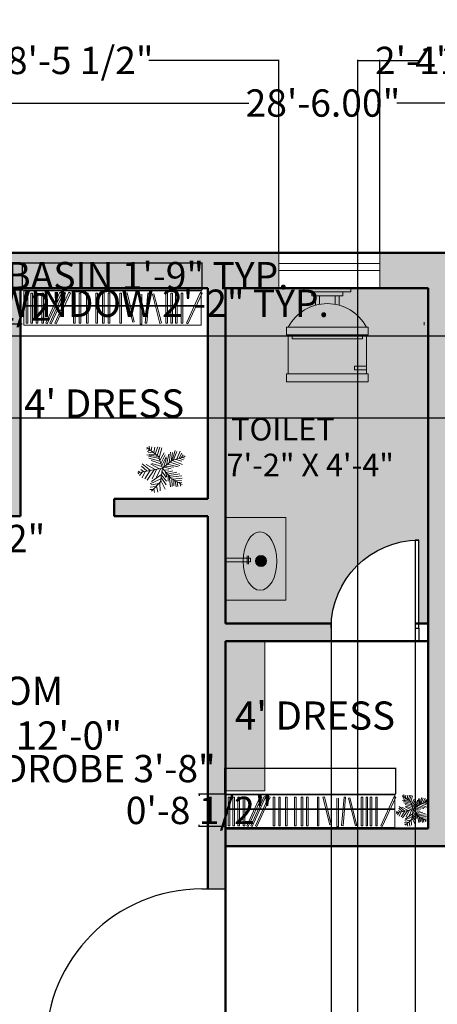
# Model space of a CAD drawing. Units: inches. Extents: x 2974 to 3443, y 2405 to 2963.
# Tile 12 of 13: x 3136 to 3243, y 2711 to 2963. Entities that reach past the tile are written whole.
import ezdxf

# ---------------------------------------------------------------- set-up
doc = ezdxf.new("R2010")
doc.units = ezdxf.units.IN
doc.header["$MEASUREMENT"] = 0
doc.layers.get('0').update_dxf_attribs({"color": 251})
for name, color, linetype, lineweight in [('A-ANNO-DIMS', 2, 'Continuous', 18), ('A-AREA-IDEN', 250, 'Continuous', 25), ('A-DOOR', 32, 'Continuous', 25), ('A-FLOR-CASE-PATT', 9, 'Continuous', 13), ('A-FLOR-FIXT', 8, 'Continuous', 20), ('A-FLOR-FIXT-PATT', 254, 'Continuous', 13), ('A-FLOR-PATT', 9, 'Continuous', 13), ('A-WALL-PATT', 252, 'Continuous', 13), ('closet', 32, 'Continuous', 20), ('greenary', 106, 'Continuous', 13), ('walls', 250, 'Continuous', 50), ('windows', 159, 'Continuous', 20)]:
    doc.layers.add(name, color=color, linetype=linetype, lineweight=lineweight)
doc.styles.get("Standard").update_dxf_attribs({"font": 'arial.ttf'})
doc.dimstyles.get("Standard").update_dxf_attribs({"dimtxt": 7, "dimasz": 0.18, "dimexe": 0.18, "dimexo": 0.0625, "dimgap": 0.09, "dimtad": 0, "dimtih": 1, "dimtoh": 1, "dimzin": 0, "dimdsep": 46, "dimlunit": 3, "dimtxsty": 'Standard', "dimcen": 0.09, "dimadec": 0, "dimazin": 0, "dimtfac": 1, "dimtofl": 0, "dimtmove": 0, "dimatfit": 3, "dimfxl": 1, "dimtolj": 1, "dimtzin": 0, "dimarcsym": 0})

# ---------------------------------------------------------------- blocks, each defined once
blk = doc.blocks.new('*U2')
for p, q in [((0, 0), (0, -6)), ((40, 0), (40, -6))]:
    blk.add_line(p, q)
blk.add_lwpolyline([(0, 0), (0, 40), (1.75, 40), (1.75, 0)], close=True)
blk.add_arc((0, 0), 40, 0, 90)
blk = doc.blocks.new('closet')
at = {"layer": 'closet'}
for p, q in [((-0.71, -5.58), (5.59, 8.19)), ((-0.23, 7.39), (-0.23, -6.57)), ((6.27, 7.88), (-0.04, -5.89)), ((5.59, 8.19), (6.27, 7.88)), ((7.92, 7.84), (8.68, 7.84)), ((7.92, 7.84), (7.92, -5.51)), ((8.68, 7.84), (8.68, -5.51)), ((10.44, 7.84), (11.2, 7.84)), ((10.44, 7.84), (10.44, -5.51)), ((11.2, 7.84), (11.2, -5.51)), ((12.45, 7.84), (13.21, 7.84)), ((12.45, 7.84), (12.45, -5.51)), ((13.21, 7.84), (13.21, -5.51)), ((14.71, 7.84), (15.47, 7.84)), ((14.71, 7.84), (14.71, -5.51)), ((15.47, 7.84), (15.47, -5.51)), ((17.44, 7.75), (18.17, 7.93)), ((17.44, 7.75), (20.73, -5.2)), ((18.17, 7.93), (21.46, -5.01)), ((23.92, 7.84), (22.75, -5.46)), ((24.67, 7.78), (23.51, -5.53)), ((23.92, 7.84), (24.67, 7.78)), ((26.09, 8.25), (26.09, -5.1)), ((26.84, 8.25), (26.84, -5.1)), ((29.49, 7.29), (32.64, -5.69)), ((30.22, 7.46), (33.37, -5.51)), ((35.23, 7.84), (35.23, -5.51)), ((35.99, 7.84), (35.99, -5.51)), ((40.33, 7.84), (40.33, -5.51)), ((41.08, 7.84), (41.08, -5.51)), ((42.85, 7.84), (42.85, -5.51)), ((43.61, 7.84), (43.61, -5.51)), ((45.9, 7.84), (45.9, -5.51)), ((46.65, 7.84), (46.65, -5.51)), ((50.07, 7.84), (50.07, -5.51)), ((50.82, 7.84), (50.82, -5.51)), ((53.32, 7.84), (53.32, -5.51)), ((54.08, 7.84), (54.08, -5.51)), ((55.9, 7.84), (55.9, -5.51)), ((56.65, 7.84), (56.65, -5.51)), ((57.99, -5.58), (64.3, 8.19)), ((64.97, 7.88), (58.67, -5.89)), ((60.19, -5.58), (66.49, 8.19)), ((67.17, 7.88), (60.87, -5.89)), ((62, -5.58), (68.3, 8.19)), ((68.98, 7.88), (62.67, -5.89)), ((69.96, 7.84), (69.96, -5.51)), ((70.72, 7.84), (70.72, -5.51)), ((72.43, 7.84), (72.43, -5.51)), ((73.19, 7.84), (73.19, -5.51)), ((74.82, 7.84), (74.82, -5.51)), ((75.57, 7.84), (75.57, -5.51)), ((76.94, 7.84), (76.94, -5.51)), ((77.69, 7.84), (77.69, -5.51)), ((56.23, 0.33), (0, 0.33)), ((56.2, 0), (0, 0)), ((56.2, 0), (78.76, 0)), ((56.23, 0.33), (78.76, 0.33)), ((-0.04, -5.89), (-0.71, -5.58)), ((21.46, -5.01), (20.73, -5.2)), ((23.51, -5.53), (22.75, -5.46)), ((33.37, -5.51), (32.64, -5.69)), ((35.99, -5.51), (35.23, -5.51)), ((41.08, -5.51), (40.33, -5.51)), ((43.61, -5.51), (42.85, -5.51)), ((46.65, -5.51), (45.9, -5.51)), ((50.82, -5.51), (50.07, -5.51)), ((54.08, -5.51), (53.32, -5.51)), ((56.65, -5.51), (55.9, -5.51)), ((58.67, -5.89), (57.99, -5.58)), ((60.87, -5.89), (60.19, -5.58)), ((62.67, -5.89), (62, -5.58)), ((70.72, -5.51), (69.96, -5.51)), ((73.19, -5.51), (72.43, -5.51)), ((75.57, -5.51), (74.82, -5.51)), ((77.69, -5.51), (76.94, -5.51))]:
    blk.add_line(p, q, dxfattribs=at)
blk = doc.blocks.new('rotated closet')
at = {"layer": 'closet'}
for p, q in [((26.32, 0.86), (27.07, 0.86)), ((29.72, -0.11), (30.45, 0.07)), ((35.46, 0.45), (36.22, 0.45)), ((40.56, 0.45), (41.31, 0.45)), ((43.08, 0.45), (43.84, 0.45)), ((46.13, 0.45), (46.88, 0.45)), ((50.3, 0.45), (51.05, 0.45)), ((53.56, 0.45), (54.31, 0.45)), ((56.13, 0.45), (56.88, 0.45)), ((64.53, 0.8), (65.2, 0.49)), ((66.72, 0.8), (67.4, 0.49)), ((68.53, 0.8), (69.21, 0.49)), ((70.19, 0.45), (70.95, 0.45)), ((72.66, 0.45), (73.42, 0.45)), ((75.05, 0.45), (75.81, 0.45)), ((77.17, 0.45), (77.92, 0.45)), ((78.99, 0), (78.99, -13.96)), ((8.91, -12.91), (8.15, -12.91)), ((11.43, -12.91), (10.67, -12.91)), ((13.44, -12.91), (12.68, -12.91)), ((15.7, -12.91), (14.94, -12.91)), ((-0.46, -14.27), (79.54, -14.27)), ((0, -13.96), (78.99, -13.96))]:
    blk.add_line(p, q, dxfattribs=at)
blk.add_blockref('closet', (0.23, -7.39), dxfattribs=at)
blk = doc.blocks.new('*U18')
for p, q in [((-10, 22), (-10, 12)), ((-10, 21), (-7, 21)), ((-7, 21), (-7, 20)), ((10, 12), (10, 22)), ((-7, 20), (-10, 20)), ((9, 13), (-9, 13)), ((-9, 13), (-9, 12)), ((9, 12), (9, 13)), ((10.5, 12), (-10.5, 12)), ((-10.5, 10), (-10.5, 12)), ((10.5, 12), (10.5, 10)), ((10.5, 10), (-10.5, 10)), ((-3, 4.4065), (-3, 2)), ((-2, 2), (-2, 4.1658)), ((2, 4.1658), (2, 2)), ((3, 2), (3, 4.4065)), ((4, 2), (-4, 2)), ((-4, 2), (-4, 1)), ((4, 1), (4, 2))]:
    blk.add_line(p, q)
for points in [[(10.5, 22), (10.5, 24), (-10.5, 24), (-10.5, 22)], [(6, 0), (6, 1), (-6, 1), (-6, 0)]]:
    blk.add_lwpolyline(points, close=True)
blk.add_arc((0, 15.3333), 11.3333, 208.0725, 331.9275)
blk = doc.blocks.new('*U13')
for p, q in [((-7.288, 39.707), (-21.778, 46.673)), ((-8.737, 47.138), (-17.069, 52.711)), ((-10.186, 53.64), (-13.084, 55.962)), ((0, 0), (-10.5, 57)), ((-9.099, 51.782), (-6.563, 55.962)), ((-7.65, 43.423), (-2.578, 49.46)), ((-5.839, 35.992), (4.667, 48.067)), ((-5.114, 27.632), (10.463, 46.673)), ((-31.5, 4.5), (-52.5, 25.5)), ((-48.585, 21.131), (-49.309, 29.026)), ((-43.513, 28.561), (-42.427, 15.558)), ((-38.442, 26.239), (-34.819, 7.663)), ((-35.544, 28.097), (-24.314, 3.947)), ((-14.533, 2.09), (-30.834, 25.31)), ((-3.665, 19.273), (-27.574, 35.527)), ((-5.114, 28.097), (-24.676, 40.636)), ((-24.314, 23.917), (-2.941, 13.7)), ((-2.941, 16.486), (8.652, 37.85)), ((-1.129, 6.734), (9.014, 26.704)), ((3.942, 1.625), (11.187, 24.381)), ((10.101, 3.483), (17.708, 26.239)), ((16.259, 5.805), (23.142, 31.348)), ((22.055, 7.198), (27.489, 32.277)), ((27, 9), (48, 36)), ((27.127, 9.056), (31.112, 35.992)), ((31.836, 30.883), (32.561, 16.486)), ((35.096, 32.741), (37.27, 22.524)), ((38.719, 34.134), (41.979, 28.561)), ((40.53, 25.775), (48.862, 24.846)), ((43.791, 29.954), (51.036, 30.883)), ((44.153, 36.456), (45.239, 32.741)), ((-47.498, 19.737), (-55.83, 18.344)), ((-40.615, 13.7), (-55.105, 10.913)), ((-33.37, 6.269), (-52.207, 5.34)), ((-28.299, 3.483), (-47.86, -5.805)), ((-21.416, 3.018), (-38.079, -8.128)), ((0, 0), (-31.5, 4.5)), ((-15.982, 2.09), (-30.11, -9.521)), ((0, 0), (-22.5, -19.5)), ((-6.563, 1.161), (-21.416, -8.128)), ((-20.691, 13.7), (-1.129, 4.876)), ((0, 0), (27, 9)), ((0, 0), (18, -22.5)), ((6.478, 1.625), (26.04, -8.592)), ((11.187, 3.483), (30.749, -5.805)), ((18.07, 5.805), (35.096, -3.483)), ((24.229, 7.663), (46.688, 1.625)), ((29.662, 12.307), (48.137, 6.269)), ((33.285, 16.486), (48.862, 10.913)), ((36.183, 19.737), (48.137, 17.88)), ((-17.431, -15.094), (-42.789, -18.809)), ((-24.314, -21.596), (-42.427, -22.06)), ((-22.5, -19.5), (-37.5, -45)), ((-15.257, -12.772), (-30.11, -12.772)), ((-20.691, -18.345), (-17.793, -44.352)), ((-6.563, -5.805), (-19.967, -9.985)), ((-17.069, -15.094), (-12.721, -40.172)), ((-13.446, -11.378), (-8.737, -32.741)), ((-9.461, -8.592), (-6.201, -23.453)), ((-4.752, -3.483), (-3.665, -14.629)), ((2.493, -3.019), (-1.491, -20.202)), ((1.769, -2.555), (24.229, -9.521)), ((5.029, -6.27), (2.131, -25.775)), ((9.014, -11.378), (3.58, -35.992)), ((14.085, -16.951), (6.478, -40.172)), ((7.565, -9.056), (32.198, -14.629)), ((18.07, -22.524), (8.289, -45.745)), ((12.274, -15.094), (36.907, -18.809)), ((16.259, -19.738), (36.183, -22.989)), ((18, -22.5), (27, -52.5)), ((18.433, -22.524), (40.53, -29.026)), ((-28.299, -29.026), (-42.789, -31.348)), ((-30.834, -34.135), (-42.427, -35.528)), ((-34.457, -39.708), (-40.978, -42.494)), ((-26.849, -26.24), (-40.253, -25.775)), ((-32.646, -36.921), (-31.921, -44.352)), ((-29.023, -30.884), (-27.936, -43.887)), ((-25.038, -23.918), (-22.865, -45.281)), ((20.244, -30.419), (15.897, -44.816)), ((19.157, -25.311), (38.719, -33.206)), ((22.78, -37.85), (19.519, -48.532)), ((21.331, -32.741), (39.081, -40.636)), ((22.78, -38.314), (34.372, -44.816)), ((24.591, -43.423), (30.749, -47.603)), ((24.591, -45.745), (23.142, -50.854)), ((26.764, -49.925), (28.213, -50.854))]:
    blk.add_line(p, q)
blk = doc.blocks.new('*D19')
at = {"layer": 'A-ANNO-DIMS', "color": 0, "lineweight": -2, "transparency": 16777216}
for p, q in [((3042.33, 2937.52), (3042.33, 2941.76)), ((3384.33, 2937.52), (3384.33, 2941.76)), ((3042.51, 2941.58), (3194.36, 2941.58)), ((3384.15, 2941.58), (3232.3, 2941.58))]:
    blk.add_line(p, q, dxfattribs=at)
at = {"layer": 'A-ANNO-DIMS', "color": 0, "transparency": 16777216}
for points in [[(3042.51, 2941.61), (3042.51, 2941.55), (3042.33, 2941.58)], [(3384.15, 2941.61), (3384.15, 2941.55), (3384.33, 2941.58)]]:
    blk.add_solid(points, dxfattribs=at)
at = {"layer": 'Defpoints', "color": 0, "transparency": 16777216}
for p in [(3384.33, 2941.58), (3042.33, 2937.45), (3384.33, 2937.45)]:
    blk.add_point(p, dxfattribs=at)
at = {"layer": 'A-ANNO-DIMS', "color": 0, "transparency": 16777216, "insert": (3213.33, 2941.58), "char_height": 7, "attachment_point": 5}
blk.add_mtext('\\A1;28\'-6.00"', dxfattribs=at)
blk = doc.blocks.new('WIN-BATH-26IN')
for p, q in [((0, 0), (0, -9)), ((25.96, 0), (0, 0)), ((0, 0), (0, -2.72)), ((25.96, -9), (25.96, 0)), ((0, -2.72), (25.96, -2.72)), ((25.96, -4.5), (0, -4.5)), ((25.96, -2.72), (25.96, -4.5)), ((0, -9), (25.96, -9))]:
    blk.add_line(p, q)
blk = doc.blocks.new('LAVATORY-WITH-TAP')
h = blk.add_hatch(color=256)
h.dxf.hatch_style = 1
edge = h.paths.add_edge_path()
edge.add_line((0.14, 0.2), (21.04, 0.2))
edge.add_line((21.04, 0.2), (21.04, 15.46))
edge.add_line((21.04, 15.46), (10.75, 15.46))
edge.add_line((10.75, 15.46), (10.75, 10.85))
edge.add_ellipse((10.01, 6.56), major_axis=(-7.48, -0.02), ratio=0.576535, start_angle=272.6137, end_angle=620.1108, ccw=False)
edge.add_line((9.8, 10.87), (9.8, 15.46))
edge.add_line((9.8, 15.46), (0.14, 15.46))
edge.add_line((0.14, 15.46), (0.14, 0.2))
h = blk.add_hatch(color=256)
h.dxf.hatch_style = 1
edge = h.paths.add_edge_path()
edge.add_ellipse((10.01, 6.56), major_axis=(-7.48, -0.02), ratio=0.576535, start_angle=272.6137, end_angle=260.1108)
edge.add_line((10.75, 10.85), (10.75, 9.83))
edge.add_line((10.75, 9.83), (11.35, 9.83))
edge.add_line((11.35, 9.83), (11.35, 9.53))
edge.add_line((11.35, 9.53), (10.75, 9.53))
edge.add_line((10.75, 9.53), (10.75, 9.04))
edge.add_line((10.75, 9.04), (9.8, 9.04))
edge.add_line((9.8, 9.04), (9.8, 10.87))
h.paths.add_polyline_path([(8.24, 6.32, -1), (11.81, 6.32, -1)], flags=16)
h.paths.add_polyline_path([(11.45, 6.32, -1), (8.6, 6.32, -1)], flags=0)
h.paths.add_polyline_path([(8.6, 6.32, 1), (11.45, 6.32, 1)], flags=0)
edge = h.paths.add_edge_path()
edge.add_line((9.8, 9.83), (10.75, 9.83))
edge.add_line((10.75, 9.83), (10.75, 10.85))
edge.add_ellipse((10.01, 6.56), major_axis=(-7.48, -0.02), ratio=0.576535, start_angle=260.1108, end_angle=272.6137)
edge.add_line((9.8, 10.87), (9.8, 9.83))
h.paths.add_polyline_path([(9.8, 9.04), (10.75, 9.04), (10.75, 9.53), (9.8, 9.53)], flags=17)
h.paths.add_polyline_path([(9.8, 9.53), (10.75, 9.53), (10.75, 9.83), (9.8, 9.83)], flags=17)
h.paths.add_polyline_path([(10.75, 9.53), (11.35, 9.53), (11.35, 9.83), (10.75, 9.83)], flags=17)
edge = h.paths.add_edge_path()
edge.add_ellipse((10.01, 6.56), major_axis=(-7.48, -0.02), ratio=0.576535, start_angle=260.1108, end_angle=272.6137, ccw=False)
edge.add_line((10.75, 10.85), (10.75, 15.46))
edge.add_line((10.75, 15.46), (9.8, 15.46))
edge.add_line((9.8, 15.46), (9.8, 10.87))
h = blk.add_hatch(color=256)
h.dxf.hatch_style = 1
h.paths.add_polyline_path([(11.45, 6.32, 1), (8.6, 6.32, 1)], flags=0)
h.paths.add_polyline_path([(11.81, 6.32, 1), (8.24, 6.32, 1)])
h.paths.add_polyline_path([(11.45, 6.32, -1), (8.6, 6.32, -1)], flags=16)
h = blk.add_hatch(color=256)
h.dxf.hatch_style = 1
h.paths.add_polyline_path([(11.45, 6.32, 1), (8.6, 6.32, 1)])
for p, q in [((0, 15.44), (0, 0)), ((9.8, 9.04), (9.8, 15.46)), ((10.75, 9.04), (10.75, 15.46)), ((21.16, 0), (21.16, 15.46)), ((9.22, 9.83), (11.35, 9.83)), ((11.35, 9.53), (9.22, 9.53)), ((9.8, 9.04), (10.75, 9.04)), ((0, 0), (21.16, 0))]:
    blk.add_line(p, q)
blk.add_circle((10.02, 6.32), 1.43)
blk.add_ellipse((10.01, 6.56), major_axis=(-7.48, -0.02), ratio=0.576535)
blk = doc.blocks.new('*D25')
at = {"layer": 'A-ANNO-DIMS', "color": 0, "lineweight": -2, "transparency": 16777216}
for p, q in [((3136.34, 2900.56), (3136.16, 2900.56)), ((3136.34, 2893.72), (3136.34, 2900.74)), ((3182.19, 2900.56), (3136.52, 2900.56)), ((3182.37, 2893.72), (3182.37, 2900.74))]:
    blk.add_line(p, q, dxfattribs=at)
at = {"layer": 'A-ANNO-DIMS', "color": 0, "transparency": 16777216}
for points in [[(3136.52, 2900.59), (3136.52, 2900.53), (3136.34, 2900.56)], [(3182.19, 2900.59), (3182.19, 2900.53), (3182.37, 2900.56)]]:
    blk.add_solid(points, dxfattribs=at)
at = {"layer": 'Defpoints', "color": 0, "transparency": 16777216}
for p in [(3136.34, 2900.56), (3136.34, 2893.66), (3182.37, 2893.66)]:
    blk.add_point(p, dxfattribs=at)
at = {"layer": 'A-ANNO-DIMS', "color": 0, "transparency": 16777216, "insert": (3093.75, 2900.56), "char_height": 7, "attachment_point": 5}
blk.add_mtext('\\A1;WARDROBE 3\'-10"', dxfattribs=at)
blk = doc.blocks.new('*D26')
at = {"layer": 'A-ANNO-DIMS', "color": 0, "lineweight": -2, "transparency": 16777216}
for p, q in [((3136.28, 2893.66), (3129.26, 2893.66)), ((3129.44, 2893.48), (3129.44, 2893.01)), ((3136.28, 2884.95), (3129.26, 2884.95)), ((3129.44, 2885.13), (3129.44, 2885.59))]:
    blk.add_line(p, q, dxfattribs=at)
at = {"layer": 'A-ANNO-DIMS', "color": 0, "transparency": 16777216}
for points in [[(3129.41, 2893.48), (3129.47, 2893.48), (3129.44, 2893.66)], [(3129.41, 2885.13), (3129.47, 2885.13), (3129.44, 2884.95)]]:
    blk.add_solid(points, dxfattribs=at)
at = {"layer": 'Defpoints', "color": 0, "transparency": 16777216}
for p in [(3136.34, 2893.66), (3129.44, 2884.95), (3136.34, 2884.95)]:
    blk.add_point(p, dxfattribs=at)
at = {"layer": 'A-ANNO-DIMS', "color": 0, "transparency": 16777216, "insert": (3129.44, 2889.3), "char_height": 7, "attachment_point": 5}
blk.add_mtext('\\A1;0\'-8 1/2"', dxfattribs=at)
blk = doc.blocks.new('*D28')
at = {"layer": 'A-ANNO-DIMS', "color": 0, "lineweight": -2, "transparency": 16777216}
for p, q in [((3111.77, 2835.69), (3120.92, 2835.69)), ((3120.74, 2835.51), (3120.74, 2833.71)), ((3120.74, 2824.49), (3120.74, 2826.29)), ((3111.77, 2824.31), (3120.92, 2824.31))]:
    blk.add_line(p, q, dxfattribs=at)
at = {"layer": 'A-ANNO-DIMS', "color": 0, "transparency": 16777216}
for points in [[(3120.71, 2835.51), (3120.77, 2835.51), (3120.74, 2835.69)], [(3120.71, 2824.49), (3120.77, 2824.49), (3120.74, 2824.31)]]:
    blk.add_solid(points, dxfattribs=at)
at = {"layer": 'Defpoints', "color": 0, "transparency": 16777216}
for p in [(3111.71, 2835.69), (3111.71, 2824.31), (3120.74, 2824.31)]:
    blk.add_point(p, dxfattribs=at)
at = {"layer": 'A-ANNO-DIMS', "color": 0, "transparency": 16777216, "insert": (3120.74, 2830), "char_height": 7, "attachment_point": 5}
blk.add_mtext('\\A1;0\'-11 1/2"', dxfattribs=at)
blk = doc.blocks.new('*D29')
at = {"layer": 'A-ANNO-DIMS', "color": 0, "lineweight": -2, "transparency": 16777216}
for p, q in [((3188.17, 2771.05), (3187.99, 2771.05)), ((3188.17, 2764.54), (3188.17, 2771.23)), ((3231.81, 2771.05), (3188.35, 2771.05)), ((3231.99, 2764.54), (3231.99, 2771.23))]:
    blk.add_line(p, q, dxfattribs=at)
at = {"layer": 'A-ANNO-DIMS', "color": 0, "transparency": 16777216}
for points in [[(3188.35, 2771.08), (3188.35, 2771.02), (3188.17, 2771.05)], [(3231.81, 2771.08), (3231.81, 2771.02), (3231.99, 2771.05)]]:
    blk.add_solid(points, dxfattribs=at)
at = {"layer": 'Defpoints', "color": 0, "transparency": 16777216}
for p in [(3188.17, 2771.05), (3188.17, 2764.48), (3231.99, 2764.48)]:
    blk.add_point(p, dxfattribs=at)
at = {"layer": 'A-ANNO-DIMS', "color": 0, "transparency": 16777216, "insert": (3148.3, 2771.05), "char_height": 7, "attachment_point": 5}
blk.add_mtext('\\A1;WARDROBE 3\'-8"', dxfattribs=at)
blk = doc.blocks.new('*D30')
at = {"layer": 'A-ANNO-DIMS', "color": 0, "lineweight": -2, "transparency": 16777216}
for p, q in [((3188.11, 2764.48), (3181.42, 2764.48)), ((3181.6, 2764.3), (3181.6, 2764.04)), ((3188.11, 2756.19), (3181.42, 2756.19)), ((3181.6, 2756.37), (3181.6, 2756.62))]:
    blk.add_line(p, q, dxfattribs=at)
at = {"layer": 'A-ANNO-DIMS', "color": 0, "transparency": 16777216}
for points in [[(3181.57, 2764.3), (3181.63, 2764.3), (3181.6, 2764.48)], [(3181.57, 2756.37), (3181.63, 2756.37), (3181.6, 2756.19)]]:
    blk.add_solid(points, dxfattribs=at)
at = {"layer": 'Defpoints', "color": 0, "transparency": 16777216}
for p in [(3188.17, 2764.48), (3181.6, 2756.19), (3188.17, 2756.19)]:
    blk.add_point(p, dxfattribs=at)
at = {"layer": 'A-ANNO-DIMS', "color": 0, "transparency": 16777216, "insert": (3181.6, 2760.33), "char_height": 7, "attachment_point": 5}
blk.add_mtext('\\A1;0\'-8 1/2"', dxfattribs=at)
blk = doc.blocks.new('*D37')
at = {"layer": 'A-ANNO-DIMS', "color": 0, "lineweight": -2, "transparency": 16777216}
for p, q in [((3074.3, 2894.13), (3074.3, 2890.11)), ((3100.26, 2894.13), (3100.26, 2890.11)), ((3074.48, 2890.29), (3100.08, 2890.29)), ((3100.26, 2890.29), (3100.44, 2890.29))]:
    blk.add_line(p, q, dxfattribs=at)
at = {"layer": 'A-ANNO-DIMS', "color": 0, "transparency": 16777216}
for points in [[(3074.48, 2890.32), (3074.48, 2890.26), (3074.3, 2890.29)], [(3100.08, 2890.32), (3100.08, 2890.26), (3100.26, 2890.29)]]:
    blk.add_solid(points, dxfattribs=at)
at = {"layer": 'Defpoints', "color": 0, "transparency": 16777216}
for p in [(3074.3, 2894.19), (3100.26, 2894.19), (3100.26, 2890.29)]:
    blk.add_point(p, dxfattribs=at)
at = {"layer": 'A-ANNO-DIMS', "color": 0, "transparency": 16777216, "insert": (3158.92, 2890.29), "char_height": 7, "attachment_point": 5}
blk.add_mtext('\\A1;BATH WINDOW 2\'-2" TYP.', dxfattribs=at)
blk = doc.blocks.new('*D41')
at = {"layer": 'A-ANNO-DIMS', "color": 0, "lineweight": -2, "transparency": 16777216}
for p, q in [((3109.7, 2894.25), (3109.7, 2897.54)), ((3109.88, 2897.36), (3130.68, 2897.36)), ((3130.86, 2894.25), (3130.86, 2897.54)), ((3130.86, 2897.36), (3131.04, 2897.36))]:
    blk.add_line(p, q, dxfattribs=at)
at = {"layer": 'A-ANNO-DIMS', "color": 0, "transparency": 16777216}
for points in [[(3109.88, 2897.39), (3109.88, 2897.33), (3109.7, 2897.36)], [(3130.68, 2897.39), (3130.68, 2897.33), (3130.86, 2897.36)]]:
    blk.add_solid(points, dxfattribs=at)
at = {"layer": 'Defpoints', "color": 0, "transparency": 16777216}
for p in [(3130.86, 2897.36), (3109.7, 2894.19), (3130.86, 2894.19)]:
    blk.add_point(p, dxfattribs=at)
at = {"layer": 'A-ANNO-DIMS', "color": 0, "transparency": 16777216, "insert": (3168.34, 2897.36), "char_height": 7, "attachment_point": 5}
blk.add_mtext('\\A1;BASIN 1\'-9" TYP.', dxfattribs=at)
blk = doc.blocks.new('*D52')
at = {"layer": 'A-ANNO-DIMS', "color": 0, "lineweight": -2, "transparency": 16777216}
for p, q in [((3100.26, 2903.25), (3100.26, 2952.68)), ((3100.44, 2952.5), (3133.57, 2952.5)), ((3201.81, 2952.5), (3168.68, 2952.5)), ((3201.99, 2903.25), (3201.99, 2952.68))]:
    blk.add_line(p, q, dxfattribs=at)
at = {"layer": 'A-ANNO-DIMS', "color": 0, "transparency": 16777216}
for points in [[(3100.44, 2952.53), (3100.44, 2952.47), (3100.26, 2952.5)], [(3201.81, 2952.53), (3201.81, 2952.47), (3201.99, 2952.5)]]:
    blk.add_solid(points, dxfattribs=at)
at = {"layer": 'Defpoints', "color": 0, "transparency": 16777216}
for p in [(3201.99, 2952.5), (3100.26, 2903.19), (3201.99, 2903.19)]:
    blk.add_point(p, dxfattribs=at)
at = {"layer": 'A-ANNO-DIMS', "color": 0, "transparency": 16777216, "insert": (3151.13, 2952.5), "char_height": 7, "attachment_point": 5}
blk.add_mtext('\\A1;8\'-5 1/2"', dxfattribs=at)
blk = doc.blocks.new('*D53')
at = {"layer": 'A-ANNO-DIMS', "color": 0, "lineweight": -2, "transparency": 16777216}
for p, q in [((3227.95, 2903.25), (3227.95, 2952.68)), ((3228.13, 2952.5), (3238.07, 2952.5)), ((3283.38, 2952.5), (3273.45, 2952.5)), ((3283.56, 2903.25), (3283.56, 2952.68))]:
    blk.add_line(p, q, dxfattribs=at)
at = {"layer": 'A-ANNO-DIMS', "color": 0, "transparency": 16777216}
for points in [[(3228.13, 2952.53), (3228.13, 2952.47), (3227.95, 2952.5)], [(3283.38, 2952.53), (3283.38, 2952.47), (3283.56, 2952.5)]]:
    blk.add_solid(points, dxfattribs=at)
at = {"layer": 'Defpoints', "color": 0, "transparency": 16777216}
for p in [(3283.56, 2952.5), (3227.95, 2903.19), (3283.56, 2903.19)]:
    blk.add_point(p, dxfattribs=at)
at = {"layer": 'A-ANNO-DIMS', "color": 0, "transparency": 16777216, "insert": (3255.76, 2952.5), "char_height": 7, "attachment_point": 5}
blk.add_mtext('\\A1;4\'-7 1/2"', dxfattribs=at)
blk = doc.blocks.new('*D61')
at = {"layer": 'A-ANNO-DIMS', "color": 0, "lineweight": -2, "transparency": 16777216}
for p, q in [((3222.29, 2555.25), (3222.29, 2952.68)), ((3222.47, 2952.5), (3227.69, 2952.5)), ((3257.25, 2952.5), (3252.03, 2952.5)), ((3257.43, 2555.25), (3257.43, 2952.68))]:
    blk.add_line(p, q, dxfattribs=at)
at = {"layer": 'A-ANNO-DIMS', "color": 0, "transparency": 16777216}
for points in [[(3222.47, 2952.53), (3222.47, 2952.47), (3222.29, 2952.5)], [(3257.25, 2952.53), (3257.25, 2952.47), (3257.43, 2952.5)]]:
    blk.add_solid(points, dxfattribs=at)
at = {"layer": 'Defpoints', "color": 0, "transparency": 16777216}
for p in [(3257.43, 2952.5), (3222.29, 2555.19), (3257.43, 2555.19)]:
    blk.add_point(p, dxfattribs=at)
at = {"layer": 'A-ANNO-DIMS', "color": 0, "transparency": 16777216, "insert": (3239.86, 2952.5), "char_height": 7, "attachment_point": 5}
blk.add_mtext('\\A1;2\'-11"', dxfattribs=at)
blk = doc.blocks.new('*D64')
at = {"layer": 'A-ANNO-DIMS', "color": 0, "lineweight": -2, "transparency": 16777216}
for p, q in [((3103.48, 2840.13), (3103.48, 2414.92)), ((3124.99, 2840.13), (3124.99, 2414.92)), ((3103.66, 2415.1), (3124.81, 2415.1)), ((3124.99, 2415.1), (3125.17, 2415.1))]:
    blk.add_line(p, q, dxfattribs=at)
at = {"layer": 'A-ANNO-DIMS', "color": 0, "transparency": 16777216}
for points in [[(3103.66, 2415.13), (3103.66, 2415.07), (3103.48, 2415.1)], [(3124.81, 2415.13), (3124.81, 2415.07), (3124.99, 2415.1)]]:
    blk.add_solid(points, dxfattribs=at)
at = {"layer": 'Defpoints', "color": 0, "transparency": 16777216}
for p in [(3103.48, 2840.19), (3124.99, 2840.19), (3124.99, 2415.1)]:
    blk.add_point(p, dxfattribs=at)
at = {"layer": 'A-ANNO-DIMS', "color": 0, "transparency": 16777216, "insert": (3142.39, 2415.1), "char_height": 7, "attachment_point": 5}
blk.add_mtext('\\A1;1\'-9 1/2"', dxfattribs=at)
blk = doc.blocks.new('*D65')
at = {"layer": 'A-ANNO-DIMS', "color": 0, "lineweight": -2, "transparency": 16777216}
for p, q in [((3215.45, 2808.13), (3215.45, 2414.92)), ((3236.95, 2808.13), (3236.95, 2414.92)), ((3215.63, 2415.1), (3236.77, 2415.1)), ((3236.95, 2415.1), (3237.13, 2415.1))]:
    blk.add_line(p, q, dxfattribs=at)
at = {"layer": 'A-ANNO-DIMS', "color": 0, "transparency": 16777216}
for points in [[(3215.63, 2415.13), (3215.63, 2415.07), (3215.45, 2415.1)], [(3236.77, 2415.13), (3236.77, 2415.07), (3236.95, 2415.1)]]:
    blk.add_solid(points, dxfattribs=at)
at = {"layer": 'Defpoints', "color": 0, "transparency": 16777216}
for p in [(3215.45, 2808.19), (3236.95, 2808.19), (3236.95, 2415.1)]:
    blk.add_point(p, dxfattribs=at)
at = {"layer": 'A-ANNO-DIMS', "color": 0, "transparency": 16777216, "insert": (3254.35, 2415.1), "char_height": 7, "attachment_point": 5}
blk.add_mtext('\\A1;1\'-9 1/2"', dxfattribs=at)
blk = doc.blocks.new('*D70')
at = {"layer": 'A-ANNO-DIMS', "color": 0, "lineweight": -2, "transparency": 16777216}
for p, q in [((3075.39, 2881.91), (3409.82, 2881.91)), ((3409.64, 2881.73), (3409.64, 2875.08)), ((3409.64, 2861.09), (3409.64, 2867.75)), ((3075.39, 2860.91), (3409.82, 2860.91))]:
    blk.add_line(p, q, dxfattribs=at)
at = {"layer": 'A-ANNO-DIMS', "color": 0, "transparency": 16777216}
for points in [[(3409.61, 2881.73), (3409.67, 2881.73), (3409.64, 2881.91)], [(3409.61, 2861.09), (3409.67, 2861.09), (3409.64, 2860.91)]]:
    blk.add_solid(points, dxfattribs=at)
at = {"layer": 'Defpoints', "color": 0, "transparency": 16777216}
for p in [(3075.33, 2881.91), (3409.64, 2881.91), (3075.33, 2860.91)]:
    blk.add_point(p, dxfattribs=at)
at = {"layer": 'A-ANNO-DIMS', "color": 0, "transparency": 16777216, "insert": (3409.64, 2871.41), "char_height": 7, "attachment_point": 5}
blk.add_mtext('\\A1;1\'-9"', dxfattribs=at)

msp = doc.modelspace()

# ---------------------------------------------------------------- hatches: boundary and pattern name
at = {"layer": 'A-FLOR-CASE-PATT'}
h = msp.add_hatch(color=256, dxfattribs=at)
h.dxf.hatch_style = 1
h.paths.add_polyline_path([(3198.401, 2803.688), (3188.326, 2803.688), (3188.326, 2765.327), (3198.401, 2765.327)])
at = {"layer": 'A-FLOR-FIXT-PATT'}
h = msp.add_hatch(color=256, dxfattribs=at)
h.dxf.hatch_style = 1
h.paths.add_polyline_path([(3204.453, 2872.188), (3224.453, 2872.188), (3224.453, 2873.188), (3221.453, 2873.188), (3221.453, 2874.188), (3224.453, 2874.188), (3224.453, 2882.188), (3223.453, 2882.188), (3223.453, 2881.188), (3205.453, 2881.188), (3205.453, 2882.188), (3204.453, 2882.188)])
h.paths.add_polyline_path([(3203.953, 2870.188), (3224.953, 2870.188), (3224.953, 2872.188), (3203.953, 2872.188)])
h.paths.add_polyline_path([(3205.453, 2881.188), (3223.453, 2881.188), (3223.453, 2882.188), (3205.453, 2882.188)], flags=17)
h.paths.add_polyline_path([(3203.953, 2882.188), (3224.953, 2882.188), (3224.953, 2884.188), (3203.953, 2884.188)])
h.paths.add_polyline_path([(3204.453, 2884.188), (3224.453, 2884.188, 0.6000022)])
h.paths.add_polyline_path([(3212.453, 2890.011, -0.0889332), (3216.453, 2890.011), (3216.453, 2892.188), (3212.453, 2892.188)])
h.paths.add_polyline_path([(3216.453, 2890.011, -0.0226287), (3217.453, 2889.784), (3217.453, 2892.188), (3216.453, 2892.188)])
h.paths.add_polyline_path([(3211.453, 2889.784, -0.0226287), (3212.453, 2890.011), (3212.453, 2892.188), (3211.453, 2892.188)])
h.paths.add_polyline_path([(3210.453, 2892.188), (3218.453, 2892.188), (3218.453, 2893.188), (3210.453, 2893.188)])
h.paths.add_polyline_path([(3208.453, 2893.188), (3220.453, 2893.188), (3220.453, 2894.188), (3208.453, 2894.188)])
h.paths.add_polyline_path([(3221.453, 2873.188), (3224.453, 2873.188), (3224.453, 2874.188), (3221.453, 2874.188)], flags=17)
at = {"layer": 'A-FLOR-PATT'}
h = msp.add_hatch(dxfattribs=at)
h.set_pattern_fill('ANGLE', color=256, scale=10)
h.set_pattern_definition([(0, (0, 0), (0, 2.75), [2, -0.75]), (90, (0, 0), (-2.75, 2e-16), [2, -0.75])])
h.paths.add_polyline_path([(3240.326, 2894.188), (3220.453, 2894.188), (3220.453, 2893.188), (3218.453, 2893.188), (3218.453, 2892.188), (3217.453, 2892.188), (3217.453, 2889.784, -0.206081), (3224.453, 2884.188), (3224.953, 2884.188), (3224.953, 2882.188), (3224.453, 2882.188), (3224.453, 2872.188), (3224.953, 2872.188), (3224.953, 2870.188), (3203.953, 2870.188), (3203.953, 2872.188), (3204.453, 2872.188), (3204.453, 2882.188), (3203.953, 2882.188), (3203.953, 2884.188), (3204.453, 2884.188, -0.206081), (3211.453, 2889.784), (3211.453, 2892.188), (3210.453, 2892.188), (3210.453, 2893.188), (3208.453, 2893.188), (3208.453, 2894.188), (3201.987, 2894.188), (3188.326, 2894.188), (3188.326, 2835.37), (3203.783, 2835.37), (3203.783, 2814.209), (3188.326, 2814.209), (3188.326, 2808.188), (3215.45, 2808.188, -0.3870418), (3236.952, 2829.559), (3236.952, 2829.581), (3237.937, 2829.581), (3237.937, 2808.188), (3240.326, 2808.188)])
h.paths.add_polyline_path([(3131.326, 2894.188), (3130.856, 2894.188), (3130.856, 2878.731), (3109.695, 2878.731), (3109.695, 2894.188), (3051.326, 2894.188), (3051.326, 2877.412), (3052.326, 2877.412), (3052.326, 2875.412), (3053.326, 2875.412), (3053.326, 2874.412), (3055.73, 2874.412, -0.206081), (3061.326, 2881.412), (3061.326, 2881.912), (3063.326, 2881.912), (3063.326, 2881.412), (3073.326, 2881.412), (3073.326, 2881.912), (3075.326, 2881.912), (3075.326, 2860.912), (3073.326, 2860.912), (3073.326, 2861.412), (3063.326, 2861.412), (3063.326, 2860.912), (3061.326, 2860.912), (3061.326, 2861.412, -0.206081), (3055.73, 2868.412), (3053.326, 2868.412), (3053.326, 2867.412), (3052.326, 2867.412), (3052.326, 2865.412), (3051.326, 2865.412), (3051.326, 2840.188), (3103.485, 2840.188, -0.3870418), (3124.986, 2861.559), (3124.986, 2861.581), (3125.971, 2861.581), (3125.971, 2840.188), (3131.326, 2840.188)])
at = {"layer": 'A-WALL-PATT'}
h = msp.add_hatch(color=256, dxfattribs=at)
h.dxf.hatch_style = 1
h.paths.add_polyline_path([(3222.294, 2555.188), (3211.826, 2555.188), (3211.826, 2657.938), (3207.326, 2657.938), (3207.326, 2555.188), (3051.326, 2555.188), (3051.326, 2583.943), (3042.326, 2583.943), (3042.326, 2471.188), (3165.027, 2471.188), (3165.027, 2480.188), (3051.326, 2480.188), (3051.326, 2550.688), (3222.294, 2550.688)])
h.paths.add_polyline_path([(3188.326, 2700.207), (3183.826, 2700.207), (3183.826, 2691.688), (3051.326, 2691.688), (3051.326, 2740.572), (3042.326, 2740.572), (3042.326, 2651.235), (3045.517, 2651.235), (3051.326, 2651.235), (3051.326, 2687.188), (3188.326, 2687.188)])
h.paths.add_polyline_path([(3051.326, 2894.188), (3074.298, 2894.188), (3074.298, 2903.188), (3042.326, 2903.188), (3042.326, 2807.864), (3045.517, 2807.864), (3051.326, 2807.864), (3051.326, 2835.688), (3103.457, 2835.688), (3103.457, 2839.066, -0.0124729), (3103.485, 2840.188), (3051.326, 2840.188)])
h.paths.add_polyline_path([(3201.987, 2903.188), (3100.263, 2903.188), (3100.263, 2894.188), (3131.326, 2894.188), (3131.326, 2835.688), (3135.826, 2835.688), (3135.826, 2894.188), (3183.826, 2894.188), (3183.826, 2840.188), (3159.826, 2840.188), (3159.826, 2835.688), (3183.826, 2835.688), (3183.826, 2740.207), (3188.326, 2740.207), (3188.326, 2803.688), (3215.422, 2803.688), (3215.422, 2807.066, -0.0124729), (3215.45, 2808.188), (3188.326, 2808.188), (3188.326, 2894.188), (3201.987, 2894.188)])
h.paths.add_polyline_path([(3283.564, 2903.188), (3227.952, 2903.188), (3227.952, 2894.188), (3240.326, 2894.188), (3240.326, 2755.688), (3188.326, 2755.688), (3188.326, 2751.188), (3244.826, 2751.188), (3244.826, 2757.188), (3244.826, 2797.188), (3244.826, 2894.188), (3283.564, 2894.188)])
h.paths.add_polyline_path([(3384.326, 2903.188), (3346.694, 2903.188), (3346.694, 2894.188), (3375.326, 2894.188), (3375.326, 2755.688), (3284.826, 2755.688), (3284.826, 2751.188), (3375.326, 2751.188), (3375.326, 2710.653), (3378.517, 2710.653), (3384.326, 2710.653)])
h.paths.add_polyline_path([(3384.326, 2643.361), (3375.326, 2643.361), (3375.326, 2609.188), (3330.003, 2609.188), (3330.003, 2604.688), (3375.326, 2604.688), (3375.326, 2480.188), (3356.49, 2480.188), (3356.49, 2471.188), (3384.326, 2471.188)])
h.paths.add_polyline_path([(3267.326, 2609.188), (3262.826, 2609.188), (3262.826, 2555.188), (3257.429, 2555.188), (3257.429, 2550.688), (3262.826, 2550.688), (3262.826, 2471.188), (3293.36, 2471.188), (3293.36, 2480.188), (3267.326, 2480.188)])
h.paths.add_polyline_path([(3275.186, 2471.188), (3268.471, 2471.188), (3268.471, 2455.229), (3268.471, 2452.413), (3275.186, 2452.413)])
h.paths.add_polyline_path([(3156.684, 2471.188), (3149.969, 2471.188), (3149.969, 2452.413), (3156.684, 2452.413)])

# ---------------------------------------------------------------- linework, layer by layer
at = {"layer": 'closet'}
for p, q in [((3182.355, 2893.656), (3136.34, 2893.656)), ((3136.659, 2893.475), (3136.659, 2885.445)), ((3136.659, 2893.475), (3182.092, 2893.475)), ((3182.092, 2893.475), (3182.092, 2884.702)), ((3136.659, 2885.445), (3136.659, 2884.702)), ((3182.092, 2884.702), (3136.659, 2884.702)), ((3239.232, 2885.445), (3239.232, 2884.702)), ((3198.401, 2765.327), (3198.401, 2803.688)), ((3188.326, 2765.327), (3188.326, 2765.327)), ((3188.326, 2765.327), (3198.401, 2765.327)), ((3231.978, 2764.477), (3188.174, 2764.477)), ((3188.478, 2764.305), (3231.728, 2764.305)), ((3231.728, 2756.661), (3231.728, 2764.305)), ((3231.728, 2764.305), (3231.728, 2755.953)), ((3188.478, 2760.14), (3188.478, 2756.308)), ((3188.478, 2756.661), (3188.478, 2755.953)), ((3231.728, 2755.953), (3188.478, 2755.953))]:
    msp.add_line(p, q, dxfattribs=at)
at = {"layer": 'walls'}
for p, q in [((3042.326, 2903.188), (3384.326, 2903.188)), ((3135.826, 2835.688), (3135.826, 2894.188)), ((3135.826, 2894.188), (3183.826, 2894.188)), ((3183.826, 2840.188), (3183.826, 2894.188)), ((3188.326, 2808.188), (3188.326, 2894.188)), ((3188.326, 2894.188), (3240.326, 2894.188)), ((3240.326, 2755.688), (3240.326, 2894.188)), ((3159.826, 2840.188), (3183.826, 2840.188)), ((3159.826, 2840.188), (3159.826, 2835.688)), ((3051.326, 2835.688), (3135.826, 2835.688)), ((3159.826, 2835.688), (3183.826, 2835.688)), ((3183.826, 2740.207), (3183.826, 2835.688)), ((3188.326, 2808.188), (3215.45, 2808.188)), ((3236.952, 2808.188), (3240.326, 2808.188)), ((3188.326, 2687.188), (3188.326, 2803.688)), ((3188.326, 2803.688), (3240.326, 2803.688)), ((3188.326, 2755.688), (3240.326, 2755.688)), ((3188.326, 2751.188), (3375.326, 2751.188))]:
    msp.add_line(p, q, dxfattribs=at)

# ---------------------------------------------------------------- block references
at = {"layer": 'A-DOOR', "xscale": -0.5628703588661903, "yscale": 0.5628703588661903, "zscale": 0.5628703588661903}
msp.add_blockref('*U2', (3237.937, 2807.066), dxfattribs=at)
at = {"layer": 'A-DOOR', "rotation": 90}
msp.add_blockref('*U2', (3182.326, 2700.207), dxfattribs=at)
at = {"layer": 'A-FLOR-FIXT'}
for name, p, rotation in [('*U18', (3214.453, 2894.188), 180), ('LAVATORY-WITH-TAP', (3203.783, 2814.209), 90.00000000000531)]:
    msp.add_blockref(name, p, dxfattribs=dict(at, rotation=rotation))
at = {"layer": 'closet', "rotation": 179.9999999992007}
for p, xscale, yscale, zscale in [((3182.092, 2885.445), 0.5751841307599156, 0.5751841307599156, 0.5751841307599156), ((3231.728, 2756.661), 0.5475492351261511, 0.5475492351261511, 0.5475492351261511)]:
    msp.add_blockref('rotated closet', p, dxfattribs=dict(at, xscale=xscale, yscale=yscale, zscale=zscale))
at = {"layer": 'greenary', "rotation": 90}
for p, xscale, yscale, zscale in [((3172.217, 2848.011), 0.1113259002009375, 0.1113259002009375, 0.1113259002009375), ((3236.443, 2760.533), 0.0762846306296744, 0.0762846306296744, 0.0762846306296744)]:
    msp.add_blockref('*U13', p, dxfattribs=dict(at, xscale=xscale, yscale=yscale, zscale=zscale))
at = {"layer": 'windows'}
msp.add_blockref('WIN-BATH-26IN', (3201.987, 2903.188), dxfattribs=at)

# ---------------------------------------------------------------- texts
at = {"layer": 'A-AREA-IDEN'}
for s, height, p in [("4' DRESS", 7.2272, (3136.761, 2860.981)), ('TOILET', 5.7816, (3189.799, 2855.125)), ('7\'-2" X 4\'-4"', 5.78159, (3188.617, 2845.95)), ('BEDROOM', 7.2272, (3098.774, 2787.376)), ("4' DRESS", 7.2272, (3190.778, 2781.018)), ('11\'-0" X 12\'-0"', 7.22716, (3097.296, 2775.906))]:
    msp.add_text(s, height=height, dxfattribs=at).set_placement(p)

# ---------------------------------------------------------------- dimensions: what is measured, and where the dimension line sits
at = {"layer": 'A-ANNO-DIMS'}
for base, p1, p2, override, picture, middle in [((3201.987, 2952.498), (3100.263, 2903.188), (3201.987, 2903.188), {"dimdec": 1, "dimlfac": 1, "dimrnd": 0, "dimzin": 1, "dimdsep": 46, "dimlunit": 4, "dimfrac": 2}, '*D52', (3151.125, 2952.498)), ((3283.564, 2952.498), (3227.952, 2903.188), (3283.564, 2903.188), {"dimdec": 1, "dimlfac": 1, "dimrnd": 0, "dimzin": 1, "dimdsep": 46, "dimlunit": 4, "dimfrac": 2}, '*D53', (3255.758, 2952.498)), ((3257.429, 2952.498), (3222.294, 2555.188), (3257.429, 2555.188), {"dimdec": 1, "dimlfac": 1, "dimrnd": 0, "dimzin": 1, "dimdsep": 46, "dimlunit": 4, "dimfrac": 2}, '*D61', (3239.861, 2952.498)), ((3384.326, 2941.584), (3042.326, 2937.454), (3384.326, 2937.454), {"dimclrd": 0, "dimclre": 0, "dimclrt": 0}, '*D19', (3213.326, 2941.584)), ((3124.986, 2415.097), (3103.485, 2840.188), (3124.986, 2840.188), {"dimdec": 1, "dimlfac": 1, "dimrnd": 0, "dimzin": 1, "dimdsep": 46, "dimlunit": 4, "dimfrac": 2}, '*D64', (3142.386, 2415.097)), ((3236.952, 2415.097), (3215.45, 2808.188), (3236.952, 2808.188), {"dimdec": 1, "dimlfac": 1, "dimrnd": 0, "dimzin": 1, "dimdsep": 46, "dimlunit": 4, "dimfrac": 2}, '*D65', (3254.352, 2415.097))]:
    dim = msp.add_linear_dim(base=base, p1=p1, p2=p2, dimstyle='Standard', override=override, dxfattribs=at)
    dim.commit()
    dim.dimension.update_dxf_attribs({"geometry": picture, "text_midpoint": middle})
for base, p1, p2, text, picture, middle in [((3100.263, 2890.294), (3074.298, 2894.188), (3100.263, 2894.188), 'BATH WINDOW <> TYP.', '*D37', (3158.923, 2890.294)), ((3130.856, 2897.363), (3109.695, 2894.188), (3130.856, 2894.188), 'BASIN <> TYP.', '*D41', (3168.337, 2897.363))]:
    dim = msp.add_linear_dim(base=base, p1=p1, p2=p2, text=text, dimstyle='Standard', override={"dimdec": 1, "dimlfac": 1, "dimrnd": 0, "dimzin": 1, "dimdsep": 46, "dimlunit": 4, "dimfrac": 2}, dxfattribs=at)
    dim.commit()
    dim.dimension.update_dxf_attribs({"geometry": picture, "text_midpoint": middle})
for base, p1, p2, picture, middle in [((3136.34, 2900.56), (3182.368, 2893.656), (3136.34, 2893.656), '*D25', (3093.75, 2900.56)), ((3188.174, 2771.05), (3231.991, 2764.477), (3188.174, 2764.477), '*D29', (3148.304, 2771.05))]:
    dim = msp.add_linear_dim(base=base, p1=p1, p2=p2, angle=180, text='WARDROBE <>', dimstyle='Standard', override={"dimdec": 1, "dimlfac": 1, "dimrnd": 0, "dimzin": 1, "dimdsep": 46, "dimlunit": 4, "dimfrac": 2}, dxfattribs=at)
    dim.commit()
    dim.dimension.update_dxf_attribs({"geometry": picture, "text_midpoint": middle})
for base, p1, p2, angle, picture, middle in [((3129.436, 2884.951), (3136.34, 2893.656), (3136.34, 2884.951), 270, '*D26', (3129.436, 2889.303)), ((3409.636, 2881.912), (3075.326, 2860.912), (3075.326, 2881.912), 90, '*D70', (3409.636, 2871.412)), ((3120.74, 2824.306), (3111.712, 2835.688), (3111.712, 2824.306), 270, '*D28', (3120.74, 2829.997)), ((3181.602, 2756.191), (3188.174, 2764.477), (3188.174, 2756.191), 270, '*D30', (3181.602, 2760.334))]:
    dim = msp.add_linear_dim(base=base, p1=p1, p2=p2, angle=angle, dimstyle='Standard', override={"dimdec": 1, "dimlfac": 1, "dimrnd": 0, "dimzin": 1, "dimdsep": 46, "dimlunit": 4, "dimfrac": 2}, dxfattribs=at)
    dim.commit()
    dim.dimension.update_dxf_attribs({"geometry": picture, "text_midpoint": middle})

doc.saveas('drawing.dxf')
